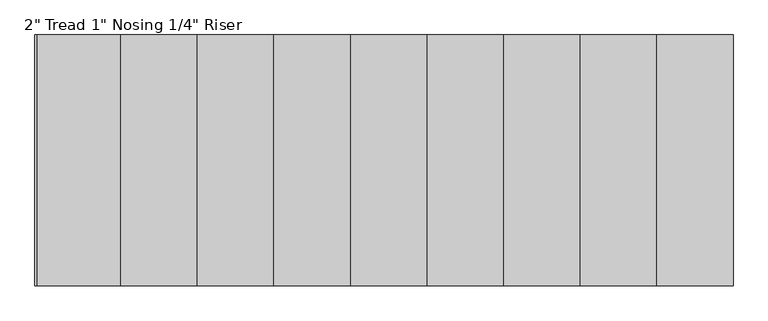
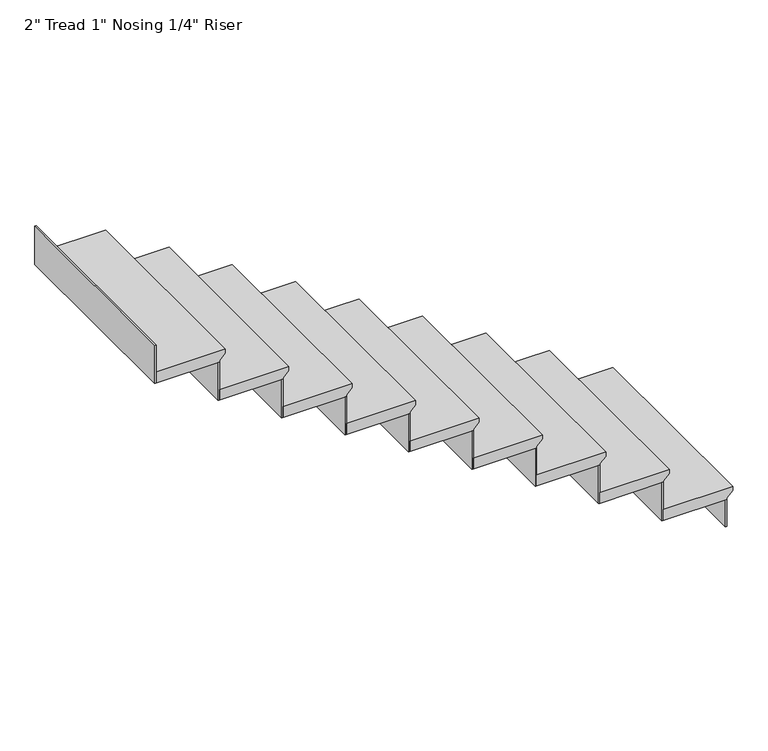
"""IFC4 building model written with IfcOpenShell, lengths in millimetres: stair flight geometry."""

from ifc_helpers import new_model, si_unit, origin, place, context, project, spatial, faceted_brep, source, transform, mapped, element, save


def stair_flight_4e768039(model_context):
    return source(origin(), model_context, "Body", "Brep", [
        faceted_brep([(-9543.8120641, -2647.9669819, 7169.15), (-9543.8120641, -2647.9669819, 7188.2), (-9543.8120641, -3562.3669819, 7188.2), (-9543.8120641, -3562.3669819, 7169.15), (-9569.2120641, -2647.9669819, 7143.75), (-9569.2120641, -3562.3669819, 7143.75), (-9848.6120641, -2647.9669819, 7188.2), (-9848.6120641, -3562.3669819, 7188.2), (-9569.2120641, -3562.3669819, 7137.4), (-9848.6120641, -3562.3669819, 7137.4), (-9848.6120641, -2647.9669819, 7137.4), (-9569.2120641, -2647.9669819, 7137.4)], [[[0, 1, 2, 3]], [[4, 0, 3, 5]], [[2, 1, 6, 7]], [[8, 9, 10, 11]], [[2, 7, 9, 8, 5, 3]], [[8, 11, 4, 5]], [[6, 1, 0, 4, 11, 10]], [[7, 6, 10, 9]]]),
        faceted_brep([(-9569.2120641, -2647.9669819, 7137.4), (-9569.2120641, -2647.9669819, 7010.4), (-9575.5620641, -2647.9669819, 7010.4), (-9575.5620641, -2647.9669819, 7137.4), (-9569.2120641, -3562.3669819, 7137.4), (-9575.5620641, -3562.3669819, 7137.4), (-9575.5620641, -3562.3669819, 7010.4), (-9569.2120641, -3562.3669819, 7010.4)], [[[0, 1, 2, 3]], [[4, 5, 6, 7]], [[1, 0, 4, 7]], [[2, 1, 7, 6]], [[3, 2, 6, 5]], [[0, 3, 5, 4]]]),
        faceted_brep([(-9848.6120641, -2647.9669819, 7315.2), (-9848.6120641, -2647.9669819, 7137.4), (-9854.9620641, -2647.9669819, 7137.4), (-9854.9620641, -2647.9669819, 7315.2), (-9848.6120641, -3562.3669819, 7315.2), (-9854.9620641, -3562.3669819, 7315.2), (-9854.9620641, -3562.3669819, 7137.4), (-9848.6120641, -3562.3669819, 7137.4)], [[[0, 1, 2, 3]], [[4, 5, 6, 7]], [[1, 0, 4, 7]], [[2, 1, 7, 6]], [[3, 2, 6, 5]], [[0, 3, 5, 4]]]),
        faceted_brep([(-9823.2120641, -3562.3669819, 7366.0), (-9823.2120641, -2647.9669819, 7366.0), (-10128.0120641, -2647.9669819, 7366.0), (-10128.0120641, -3562.3669819, 7366.0), (-9848.6120641, -3562.3669819, 7315.2), (-10128.0120641, -3562.3669819, 7315.2), (-10128.0120641, -2647.9669819, 7315.2), (-9848.6120641, -2647.9669819, 7315.2), (-9848.6120641, -3562.3669819, 7321.55), (-9823.2120641, -3562.3669819, 7346.95), (-9848.6120641, -2647.9669819, 7321.55), (-9823.2120641, -2647.9669819, 7346.95)], [[[0, 1, 2, 3]], [[4, 5, 6, 7]], [[0, 3, 5, 4, 8, 9]], [[4, 7, 10, 8]], [[2, 1, 11, 10, 7, 6]], [[3, 2, 6, 5]], [[11, 1, 0, 9]], [[10, 11, 9, 8]]]),
        faceted_brep([(-10128.0120641, -2647.9669819, 7493.0), (-10128.0120641, -2647.9669819, 7315.2), (-10134.3620641, -2647.9669819, 7315.2), (-10134.3620641, -2647.9669819, 7493.0), (-10128.0120641, -3562.3669819, 7493.0), (-10134.3620641, -3562.3669819, 7493.0), (-10134.3620641, -3562.3669819, 7315.2), (-10128.0120641, -3562.3669819, 7315.2)], [[[0, 1, 2, 3]], [[4, 5, 6, 7]], [[1, 0, 4, 7]], [[2, 1, 7, 6]], [[3, 2, 6, 5]], [[0, 3, 5, 4]]]),
        faceted_brep([(-10102.6120641, -3562.3669819, 7543.8), (-10102.6120641, -2647.9669819, 7543.8), (-10407.4120641, -2647.9669819, 7543.8), (-10407.4120641, -3562.3669819, 7543.8), (-10128.0120641, -3562.3669819, 7493.0), (-10407.4120641, -3562.3669819, 7493.0), (-10407.4120641, -2647.9669819, 7493.0), (-10128.0120641, -2647.9669819, 7493.0), (-10128.0120641, -3562.3669819, 7499.35), (-10102.6120641, -3562.3669819, 7524.75), (-10128.0120641, -2647.9669819, 7499.35), (-10102.6120641, -2647.9669819, 7524.75)], [[[0, 1, 2, 3]], [[4, 5, 6, 7]], [[0, 3, 5, 4, 8, 9]], [[4, 7, 10, 8]], [[2, 1, 11, 10, 7, 6]], [[3, 2, 6, 5]], [[11, 1, 0, 9]], [[10, 11, 9, 8]]]),
        faceted_brep([(-10407.4120641, -2647.9669819, 7670.8), (-10407.4120641, -2647.9669819, 7493.0), (-10413.7620641, -2647.9669819, 7493.0), (-10413.7620641, -2647.9669819, 7670.8), (-10407.4120641, -3562.3669819, 7670.8), (-10413.7620641, -3562.3669819, 7670.8), (-10413.7620641, -3562.3669819, 7493.0), (-10407.4120641, -3562.3669819, 7493.0)], [[[0, 1, 2, 3]], [[4, 5, 6, 7]], [[1, 0, 4, 7]], [[2, 1, 7, 6]], [[3, 2, 6, 5]], [[0, 3, 5, 4]]]),
        faceted_brep([(-10382.0120641, -3562.3669819, 7721.6), (-10382.0120641, -2647.9669819, 7721.6), (-10686.8120641, -2647.9669819, 7721.6), (-10686.8120641, -3562.3669819, 7721.6), (-10407.4120641, -3562.3669819, 7670.8), (-10686.8120641, -3562.3669819, 7670.8), (-10686.8120641, -2647.9669819, 7670.8), (-10407.4120641, -2647.9669819, 7670.8), (-10407.4120641, -3562.3669819, 7677.15), (-10382.0120641, -3562.3669819, 7702.55), (-10407.4120641, -2647.9669819, 7677.15), (-10382.0120641, -2647.9669819, 7702.55)], [[[0, 1, 2, 3]], [[4, 5, 6, 7]], [[0, 3, 5, 4, 8, 9]], [[4, 7, 10, 8]], [[2, 1, 11, 10, 7, 6]], [[3, 2, 6, 5]], [[11, 1, 0, 9]], [[10, 11, 9, 8]]]),
        faceted_brep([(-10686.8120641, -2647.9669819, 7848.6), (-10686.8120641, -2647.9669819, 7670.8), (-10693.1620641, -2647.9669819, 7670.8), (-10693.1620641, -2647.9669819, 7848.6), (-10686.8120641, -3562.3669819, 7848.6), (-10693.1620641, -3562.3669819, 7848.6), (-10693.1620641, -3562.3669819, 7670.8), (-10686.8120641, -3562.3669819, 7670.8)], [[[0, 1, 2, 3]], [[4, 5, 6, 7]], [[1, 0, 4, 7]], [[2, 1, 7, 6]], [[3, 2, 6, 5]], [[0, 3, 5, 4]]]),
        faceted_brep([(-10661.4120641, -3562.3669819, 7899.4), (-10661.4120641, -2647.9669819, 7899.4), (-10966.2120641, -2647.9669819, 7899.4), (-10966.2120641, -3562.3669819, 7899.4), (-10686.8120641, -3562.3669819, 7848.6), (-10966.2120641, -3562.3669819, 7848.6), (-10966.2120641, -2647.9669819, 7848.6), (-10686.8120641, -2647.9669819, 7848.6), (-10686.8120641, -3562.3669819, 7854.95), (-10661.4120641, -3562.3669819, 7880.35), (-10686.8120641, -2647.9669819, 7854.95), (-10661.4120641, -2647.9669819, 7880.35)], [[[0, 1, 2, 3]], [[4, 5, 6, 7]], [[0, 3, 5, 4, 8, 9]], [[4, 7, 10, 8]], [[2, 1, 11, 10, 7, 6]], [[3, 2, 6, 5]], [[11, 1, 0, 9]], [[10, 11, 9, 8]]]),
        faceted_brep([(-10966.2120641, -2647.9669819, 8026.4), (-10966.2120641, -2647.9669819, 7848.6), (-10972.5620641, -2647.9669819, 7848.6), (-10972.5620641, -2647.9669819, 8026.4), (-10966.2120641, -3562.3669819, 8026.4), (-10972.5620641, -3562.3669819, 8026.4), (-10972.5620641, -3562.3669819, 7848.6), (-10966.2120641, -3562.3669819, 7848.6)], [[[0, 1, 2, 3]], [[4, 5, 6, 7]], [[1, 0, 4, 7]], [[2, 1, 7, 6]], [[3, 2, 6, 5]], [[0, 3, 5, 4]]]),
        faceted_brep([(-10940.8120641, -3562.3669819, 8077.2), (-10940.8120641, -2647.9669819, 8077.2), (-11245.6120641, -2647.9669819, 8077.2), (-11245.6120641, -3562.3669819, 8077.2), (-10966.2120641, -3562.3669819, 8026.4), (-11245.6120641, -3562.3669819, 8026.4), (-11245.6120641, -2647.9669819, 8026.4), (-10966.2120641, -2647.9669819, 8026.4), (-10966.2120641, -3562.3669819, 8032.75), (-10940.8120641, -3562.3669819, 8058.15), (-10966.2120641, -2647.9669819, 8032.75), (-10940.8120641, -2647.9669819, 8058.15)], [[[0, 1, 2, 3]], [[4, 5, 6, 7]], [[0, 3, 5, 4, 8, 9]], [[4, 7, 10, 8]], [[2, 1, 11, 10, 7, 6]], [[3, 2, 6, 5]], [[11, 1, 0, 9]], [[10, 11, 9, 8]]]),
        faceted_brep([(-11245.6120641, -2647.9669819, 8204.2), (-11245.6120641, -2647.9669819, 8026.4), (-11251.9620641, -2647.9669819, 8026.4), (-11251.9620641, -2647.9669819, 8204.2), (-11245.6120641, -3562.3669819, 8204.2), (-11251.9620641, -3562.3669819, 8204.2), (-11251.9620641, -3562.3669819, 8026.4), (-11245.6120641, -3562.3669819, 8026.4)], [[[0, 1, 2, 3]], [[4, 5, 6, 7]], [[1, 0, 4, 7]], [[2, 1, 7, 6]], [[3, 2, 6, 5]], [[0, 3, 5, 4]]]),
        faceted_brep([(-11220.2120641, -3562.3669819, 8255.0), (-11220.2120641, -2647.9669819, 8255.0), (-11525.0120641, -2647.9669819, 8255.0), (-11525.0120641, -3562.3669819, 8255.0), (-11245.6120641, -3562.3669819, 8204.2), (-11525.0120641, -3562.3669819, 8204.2), (-11525.0120641, -2647.9669819, 8204.2), (-11245.6120641, -2647.9669819, 8204.2), (-11245.6120641, -3562.3669819, 8210.55), (-11220.2120641, -3562.3669819, 8235.95), (-11245.6120641, -2647.9669819, 8210.55), (-11220.2120641, -2647.9669819, 8235.95)], [[[0, 1, 2, 3]], [[4, 5, 6, 7]], [[0, 3, 5, 4, 8, 9]], [[4, 7, 10, 8]], [[2, 1, 11, 10, 7, 6]], [[3, 2, 6, 5]], [[11, 1, 0, 9]], [[10, 11, 9, 8]]]),
        faceted_brep([(-11525.0120641, -2647.9669819, 8382.0), (-11525.0120641, -2647.9669819, 8204.2), (-11531.3620641, -2647.9669819, 8204.2), (-11531.3620641, -2647.9669819, 8382.0), (-11525.0120641, -3562.3669819, 8382.0), (-11531.3620641, -3562.3669819, 8382.0), (-11531.3620641, -3562.3669819, 8204.2), (-11525.0120641, -3562.3669819, 8204.2)], [[[0, 1, 2, 3]], [[4, 5, 6, 7]], [[1, 0, 4, 7]], [[2, 1, 7, 6]], [[3, 2, 6, 5]], [[0, 3, 5, 4]]]),
        faceted_brep([(-11499.6120641, -3562.3669819, 8432.8), (-11499.6120641, -2647.9669819, 8432.8), (-11804.4120641, -2647.9669819, 8432.8), (-11804.4120641, -3562.3669819, 8432.8), (-11525.0120641, -3562.3669819, 8382.0), (-11804.4120641, -3562.3669819, 8382.0), (-11804.4120641, -2647.9669819, 8382.0), (-11525.0120641, -2647.9669819, 8382.0), (-11525.0120641, -3562.3669819, 8388.35), (-11499.6120641, -3562.3669819, 8413.75), (-11525.0120641, -2647.9669819, 8388.35), (-11499.6120641, -2647.9669819, 8413.75)], [[[0, 1, 2, 3]], [[4, 5, 6, 7]], [[0, 3, 5, 4, 8, 9]], [[4, 7, 10, 8]], [[2, 1, 11, 10, 7, 6]], [[3, 2, 6, 5]], [[11, 1, 0, 9]], [[10, 11, 9, 8]]]),
        faceted_brep([(-12083.8120641, -2647.9669819, 8737.6), (-12083.8120641, -2647.9669819, 8559.8), (-12090.1620641, -2647.9669819, 8559.8), (-12090.1620641, -2647.9669819, 8737.6), (-12083.8120641, -3562.3669819, 8737.6), (-12090.1620641, -3562.3669819, 8737.6), (-12090.1620641, -3562.3669819, 8559.8), (-12083.8120641, -3562.3669819, 8559.8)], [[[0, 1, 2, 3]], [[4, 5, 6, 7]], [[1, 0, 4, 7]], [[2, 1, 7, 6]], [[3, 2, 6, 5]], [[0, 3, 5, 4]]]),
        faceted_brep([(-11804.4120641, -2647.9669819, 8559.8), (-11804.4120641, -2647.9669819, 8382.0), (-11810.7620641, -2647.9669819, 8382.0), (-11810.7620641, -2647.9669819, 8559.8), (-11804.4120641, -3562.3669819, 8559.8), (-11810.7620641, -3562.3669819, 8559.8), (-11810.7620641, -3562.3669819, 8382.0), (-11804.4120641, -3562.3669819, 8382.0)], [[[0, 1, 2, 3]], [[4, 5, 6, 7]], [[1, 0, 4, 7]], [[2, 1, 7, 6]], [[3, 2, 6, 5]], [[0, 3, 5, 4]]]),
        faceted_brep([(-11779.0120641, -3562.3669819, 8610.6), (-11779.0120641, -2647.9669819, 8610.6), (-12058.4120641, -2647.9669819, 8610.6), (-12083.8120641, -2647.9669819, 8610.6), (-12083.8120641, -3562.3669819, 8610.6), (-11804.4120641, -3562.3669819, 8559.8), (-12083.8120641, -3562.3669819, 8559.8), (-12083.8120641, -2647.9669819, 8559.8), (-12058.4120641, -2647.9669819, 8559.8), (-11804.4120641, -2647.9669819, 8559.8), (-11804.4120641, -3562.3669819, 8566.15), (-11779.0120641, -3562.3669819, 8591.55), (-11804.4120641, -2647.9669819, 8566.15), (-11779.0120641, -2647.9669819, 8591.55)], [[[0, 1, 2, 3, 4]], [[5, 6, 7, 8, 9]], [[0, 4, 6, 5, 10, 11]], [[5, 9, 12, 10]], [[2, 1, 13, 12, 9, 8]], [[3, 2, 8, 7]], [[4, 3, 7, 6]], [[13, 1, 0, 11]], [[12, 13, 11, 10]]]),
    ])


if __name__ == "__main__":
    model = new_model("IFC4")
    model_context = context("Model", 3, world=origin())
    ifc_project = project(units=[si_unit("LENGTHUNIT", "METRE", prefix="MILLI")], contexts=[model_context])
    site = spatial("IfcSite", under=ifc_project)
    building = spatial("IfcBuilding", under=site)
    placement = place(None, origin())
    stair_flight_shape = stair_flight_4e768039(model_context)
    element("IfcStairFlight", 1, ObjectType="2\" Tread 1\" Nosing 1/4\" Riser", at=placement, inside=building, context=model_context, shape_type="MappedRepresentation", body=[
        mapped(stair_flight_shape, transform((0.0, 0.0, 0.0), x_axis=(1.0, 0.0, 0.0), y_axis=(0.0, 1.0, 0.0), z_axis=(0.0, 0.0, 1.0))),
    ])
    save(model, "model.ifc")
